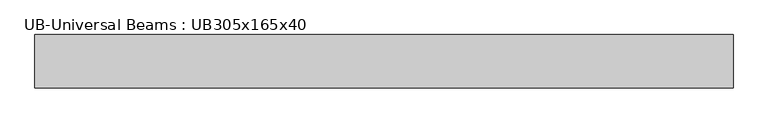
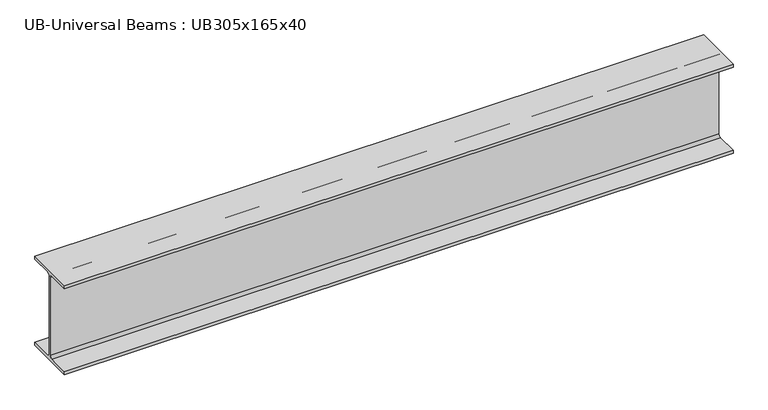
"""IFC4 building model written with IfcOpenShell, lengths in millimetres: beam geometry, UB-Universal Beams : UB305x165x40."""

from ifc_helpers import new_model, si_unit, point, frame, frame_2d, origin, place, context, project, spatial, polyline, circle_curve, trimmed, segment, composite_curve, outline, extrude, source, transform, mapped, element, save


def ub_universal_beams_ub305x165x40_46a3dc55(model_context):
    return source(origin(), model_context, "Body", "SweptSolid", [
        extrude(outline(composite_curve([segment(polyline([(82.5, -141.5), (82.5, -151.7), (-82.5, -151.7), (-82.5, -141.5), (-11.9, -141.5)]), True, "CONTINUOUS"), segment(trimmed(circle_curve(frame_2d((-11.9, -132.6)), 8.9), [point((-11.9, -141.5))], [point((-3.0, -132.6))], True, "CARTESIAN"), True, "CONTINUOUS"), segment(polyline([(-3.0, -132.6), (-3.0, 132.6)]), True, "CONTINUOUS"), segment(trimmed(circle_curve(frame_2d((-11.9, 132.6)), 8.9), [point((-3.0, 132.6))], [point((-11.9, 141.5))], True, "CARTESIAN"), True, "CONTINUOUS"), segment(polyline([(-11.9, 141.5), (-82.5, 141.5), (-82.5, 151.7), (82.5, 151.7), (82.5, 141.5), (11.9, 141.5)]), True, "CONTINUOUS"), segment(trimmed(circle_curve(frame_2d((11.9, 132.6)), 8.9), [point((11.9, 141.5))], [point((3.0, 132.6))], True, "CARTESIAN"), True, "CONTINUOUS"), segment(polyline([(3.0, 132.6), (3.0, -132.6)]), True, "CONTINUOUS"), segment(trimmed(circle_curve(frame_2d((11.9, -132.6)), 8.9), [point((3.0, -132.6))], [point((11.9, -141.5))], True, "CARTESIAN"), True, "CONTINUOUS"), segment(polyline([(11.9, -141.5), (82.5, -141.5)]), True, "CONTINUOUS")], self_intersect=False)), frame((-1564.0, 0.0, 0.0), z_axis=(1.0, 0.0, 0.0), x_axis=(0.0, 1.0, 0.0)), (0.0, 0.0, 1.0), 2152.8),
    ])


if __name__ == "__main__":
    model = new_model("IFC4")
    model_context = context("Model", 3, world=origin())
    ifc_project = project(units=[si_unit("LENGTHUNIT", "METRE", prefix="MILLI")], contexts=[model_context])
    site = spatial("IfcSite", under=ifc_project)
    building = spatial("IfcBuilding", under=site)
    placement = place(None, origin())
    ub_universal_beams_ub305x165x40_shape = ub_universal_beams_ub305x165x40_46a3dc55(model_context)
    element("IfcBeam", 1, ObjectType="UB-Universal Beams : UB305x165x40", at=placement, inside=building, context=model_context, shape_type="MappedRepresentation", body=[
        mapped(ub_universal_beams_ub305x165x40_shape, transform((0.0, 0.0, 0.0), x_axis=(1.0, 0.0, 0.0), y_axis=(0.0, 1.0, 0.0), z_axis=(0.0, 0.0, 1.0))),
    ])
    save(model, "model.ifc")

# Revit data of these elements
# Type "UB-Universal Beams : UB305x165x40"
#   Section Name Key = "UB305X165X40"
#   Width = 16.5 cm
#   Web Thickness = 0.6 cm
#   Web Fillet = 0.89 cm
#   Warping Constant = 164000.0 cm⁶
#   Torsional Moment of Inertia = 14.70 cm⁴
#   Section Area = 51.3 cm²
#   Plastic Modulus weak axis = 142.0 cm³
#   Plastic Modulus strong axis = 623.0 cm³
#   Nominal Weight = 40.2999 kgf/m
#   Moment of Inertia weak axis = 764.00 cm⁴
#   Moment of Inertia strong axis = 8503.00 cm⁴
#   Height = 30.34 cm
#   Flange Thickness = 1.02 cm
#   Elastic Modulus weak axis = 92.6 cm³
#   Elastic Modulus strong axis = 560.0 cm³
#   Centroid Vertical = 15.17 cm
#   Centroid Horizontal = 8.25 cm
#   Bolt Spacing = 9.0 cm
#   Length [instance default] = 1500 mm
#   Structural Material [instance default] = Metal - Steel 43-275
#   Type Comments = ""
#   Assembly Code = ""
# Element 1 (IfcBeam, "UB-Universal Beams : UB305x165x40")
#   Materials on its faces: "Metal - Steel 43-275"
# Materials
#   "Metal - Steel 43-275": class "Metal", colour RGB 247 247 247, transparency 0, Cost = 0
